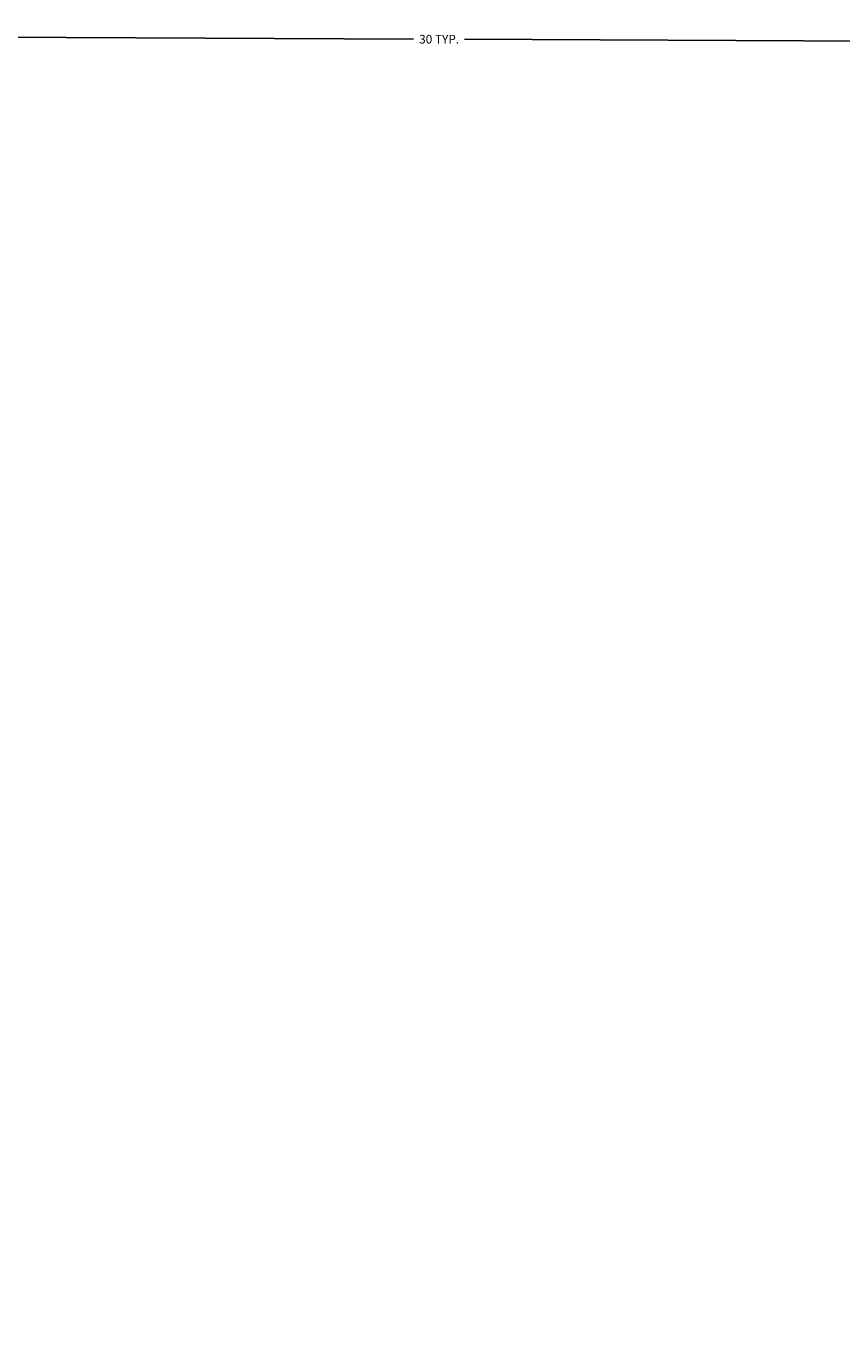
# Model space of a CAD drawing. Units: inches. Extents: x 1901 to 2863, y 888 to 2433.
# Tile 30 of 91: x 2573 to 2590, y 1376 to 1404. Entities that reach past the tile are written whole.
import ezdxf

# ---------------------------------------------------------------- set-up
doc = ezdxf.new("R2010")
doc.units = ezdxf.units.IN
doc.layers.add('A-ANNO-DIMS', color=2, linetype='Continuous', lineweight=18)
doc.layers.add('A-DOOR', color=4, linetype='Continuous', lineweight=25)
doc.styles.get("Standard").update_dxf_attribs({"font": 'arial.ttf'})
doc.dimstyles.get("Standard").update_dxf_attribs({"dimtxt": 0.18, "dimasz": 0.18, "dimexe": 0.18, "dimexo": 0.0625, "dimgap": 0.09, "dimtad": 0, "dimtih": 1, "dimtoh": 1, "dimdec": 4, "dimzin": 0, "dimdsep": 46, "dimtxsty": 'Standard', "dimcen": 0.09, "dimadec": 0, "dimazin": 0, "dimtfac": 1, "dimtdec": 4, "dimtofl": 0, "dimtmove": 0, "dimatfit": 3, "dimfxl": 1, "dimtolj": 1, "dimtzin": 0, "dimarcsym": 0})

# ---------------------------------------------------------------- blocks, each defined once
blk = doc.blocks.new('DOOR-29')
blk.add_arc((-0.004, 7.119), 28.865, 345.6888, 90)
blk = doc.blocks.new('*D32')
at = {"layer": 'A-ANNO-DIMS', "color": 0, "lineweight": -2, "transparency": 16777216}
for p, q in [((2566.833, 1398.027), (2566.858, 1403.544)), ((2567.038, 1403.364), (2581.416, 1403.297)), ((2596.85, 1403.225), (2582.472, 1403.292)), ((2597.005, 1397.887), (2597.03, 1403.404))]:
    blk.add_line(p, q, dxfattribs=at)
at = {"layer": 'A-ANNO-DIMS', "color": 0, "transparency": 16777216}
for points in [[(2567.038, 1403.394), (2567.037, 1403.334), (2566.858, 1403.364)], [(2596.85, 1403.255), (2596.849, 1403.195), (2597.03, 1403.224)]]:
    blk.add_solid(points, dxfattribs=at)
at = {"layer": 'Defpoints', "color": 0, "transparency": 16777216}
for p in [(2566.858, 1403.364), (2566.833, 1397.964), (2597.005, 1397.824)]:
    blk.add_point(p, dxfattribs=at)
at = {"layer": 'A-ANNO-DIMS', "color": 0, "transparency": 16777216, "insert": (2581.944, 1403.294), "char_height": 0.18, "attachment_point": 5}
blk.add_mtext('\\A1;30 TYP.', dxfattribs=at)

msp = doc.modelspace()

# ---------------------------------------------------------------- block references
at = {"layer": 'A-DOOR', "rotation": 179.7338121645225}
msp.add_blockref('DOOR-29', (2597.001, 1397.808), dxfattribs=at)

# ---------------------------------------------------------------- dimensions: what is measured, and where the dimension line sits
at = {"layer": 'A-ANNO-DIMS'}
dim = msp.add_linear_dim(base=(2566.858, 1403.364), p1=(2597.005, 1397.824), p2=(2566.833, 1397.964), angle=179.7338, text='<> TYP.', dimstyle='Standard', override={"dimdec": 0, "dimlfac": 1, "dimrnd": 0, "dimzin": 0, "dimdsep": 46, "dimlunit": 2}, dxfattribs=at)
dim.commit()
dim.dimension.update_dxf_attribs({"geometry": '*D32', "text_midpoint": (2581.944, 1403.294)})

doc.saveas('drawing.dxf')
